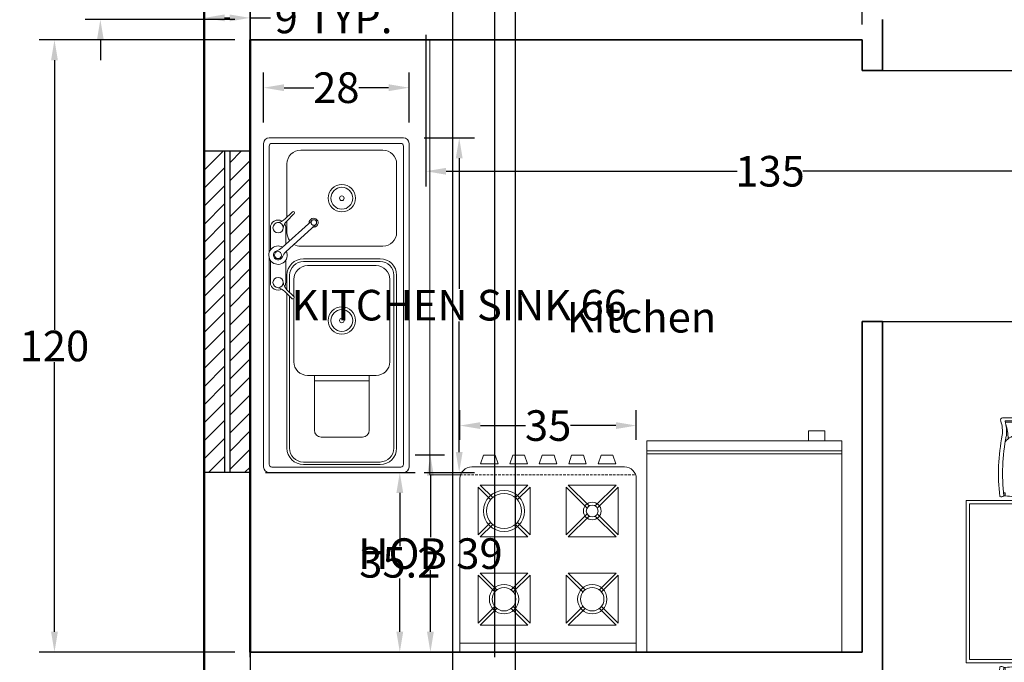
# Model space of a CAD drawing. Units: inches. Extents: x -1285 to -837, y -84 to 552.
# Tile 2 of 10: x -1282 to -1089, y 38 to 164. Entities that reach past the tile are written whole.
import ezdxf

# ---------------------------------------------------------------- set-up
doc = ezdxf.new("R2010")
doc.units = ezdxf.units.IN
doc.header["$MEASUREMENT"] = 0
doc.linetypes.add('DASHED', pattern=[0.75, 0.5, -0.25])
for name, color, linetype, lineweight in [('A-ANNO-DIMS', 2, 'Continuous', 18), ('A-AREA-IDEN', 7, 'Continuous', 25), ('A-FURN-CSWK', 9, 'Continuous', 18), ('A-FURN-CSWK-HIDN', 9, 'DASHED', 13), ('A-GLAZ-PATT', 191, 'Continuous', 13), ('Dining Table', 52, 'Continuous', 18), ('Gas Stove', 31, 'Continuous', 18), ('Inner Wall', 202, 'Continuous', 35), ('Outer Wall', 12, 'Continuous', 50), ('Refrigerator', 8, 'Continuous', 18), ('Sink', 33, 'Continuous', 18), ('Windows', 191, 'Continuous', 25)]:
    doc.layers.add(name, color=color, linetype=linetype, lineweight=lineweight)
doc.styles.get("Standard").update_dxf_attribs({"font": 'arial.ttf'})
doc.dimstyles.get("Standard").update_dxf_attribs({"dimtxt": 6, "dimasz": 4, "dimexe": 3, "dimexo": 3, "dimgap": 0.09, "dimtad": 0, "dimtih": 1, "dimtoh": 1, "dimdec": 1, "dimzin": 0, "dimdsep": 46, "dimlunit": 3, "dimtxsty": 'Standard', "dimcen": 0.09, "dimadec": 0, "dimazin": 0, "dimtfac": 1, "dimtdec": 1, "dimtofl": 0, "dimtmove": 0, "dimatfit": 3, "dimfxl": 1, "dimtolj": 1, "dimtzin": 0, "dimarcsym": 0})

# ---------------------------------------------------------------- blocks, each defined once
blk = doc.blocks.new('Gas Stove')
at = {"color": 0}
for p, q in [((1658.63, 622.25), (1657.94, 620.18)), ((1658.63, 622.25), (1661.39, 622.25)), ((1661.39, 622.25), (1662.08, 620.18)), ((1665.52, 622.25), (1664.83, 620.18)), ((1665.52, 622.25), (1668.27, 622.25)), ((1668.27, 622.25), (1668.96, 620.18)), ((1672.4, 622.25), (1671.72, 620.18)), ((1672.4, 622.25), (1675.16, 622.25)), ((1675.16, 622.25), (1675.85, 620.18)), ((1679.29, 622.25), (1678.6, 620.18)), ((1679.29, 622.25), (1682.04, 622.25)), ((1682.04, 622.25), (1682.73, 620.18)), ((1686.18, 622.25), (1685.49, 620.18)), ((1686.18, 622.25), (1688.93, 622.25)), ((1688.93, 622.25), (1689.62, 620.18)), ((1655.88, 619.49), (1691.68, 619.49)), ((1657.94, 620.18), (1662.08, 620.18)), ((1664.83, 620.18), (1668.96, 620.18)), ((1671.72, 620.18), (1675.85, 620.18)), ((1678.6, 620.18), (1682.73, 620.18)), ((1685.49, 620.18), (1689.62, 620.18)), ((1653.12, 576.11), (1653.12, 616.74)), ((1694.44, 616.74), (1694.44, 576.11)), ((1657.37, 603.57), (1657.37, 614.76)), ((1660.3, 611.83), (1657.37, 614.76)), ((1657.85, 615.25), (1669.05, 615.25)), ((1660.79, 612.32), (1657.85, 615.25)), ((1666.12, 612.32), (1669.05, 615.25)), ((1666.61, 611.83), (1669.54, 614.76)), ((1669.54, 614.76), (1669.54, 603.57)), ((1678.02, 603.57), (1678.02, 614.76)), ((1678.02, 614.76), (1682.92, 609.86)), ((1678.51, 615.25), (1689.71, 615.25)), ((1678.51, 615.25), (1683.41, 610.35)), ((1684.81, 610.35), (1689.71, 615.25)), ((1685.3, 609.86), (1690.2, 614.76)), ((1690.2, 614.76), (1690.2, 603.57)), ((1678.02, 603.57), (1682.92, 608.47)), ((1678.51, 603.08), (1683.41, 607.98)), ((1684.81, 607.98), (1689.71, 603.08)), ((1685.3, 608.47), (1690.2, 603.57)), ((1657.37, 603.57), (1660.3, 606.5)), ((1657.85, 603.08), (1660.79, 606.01)), ((1669.05, 603.08), (1666.12, 606.01)), ((1669.54, 603.57), (1666.61, 606.5)), ((1669.05, 603.08), (1657.85, 603.08)), ((1689.71, 603.08), (1678.51, 603.08)), ((1657.37, 582.91), (1657.37, 594.11)), ((1661.28, 590.2), (1657.37, 594.11)), ((1657.85, 594.59), (1669.05, 594.59)), ((1661.76, 590.68), (1657.85, 594.59)), ((1669.05, 594.59), (1665.14, 590.68)), ((1669.54, 594.11), (1665.63, 590.2)), ((1669.54, 594.11), (1669.54, 582.91)), ((1678.02, 582.91), (1678.02, 594.11)), ((1678.02, 594.11), (1681.93, 590.2)), ((1678.51, 594.59), (1689.71, 594.59)), ((1678.51, 594.59), (1682.42, 590.68)), ((1689.71, 594.59), (1685.8, 590.68)), ((1690.2, 594.11), (1686.29, 590.2)), ((1690.2, 594.11), (1690.2, 582.91)), ((1661.28, 586.82), (1657.37, 582.91)), ((1661.76, 586.33), (1657.85, 582.42)), ((1669.05, 582.42), (1665.14, 586.33)), ((1669.54, 582.91), (1665.63, 586.82)), ((1681.93, 586.82), (1678.02, 582.91)), ((1682.42, 586.33), (1678.51, 582.42)), ((1685.8, 586.33), (1689.71, 582.42)), ((1686.29, 586.82), (1690.2, 582.91)), ((1669.05, 582.42), (1657.85, 582.42)), ((1689.71, 582.42), (1678.51, 582.42)), ((1694.44, 578.18), (1653.12, 578.18)), ((1694.44, 576.11), (1653.12, 576.11))]:
    blk.add_line(p, q, dxfattribs=at)
for centre, radius in [((1663.45, 609.16), 4.82), ((1663.45, 609.16), 4.13), ((1684.11, 609.16), 2.07), ((1684.11, 609.16), 1.38), ((1663.45, 588.51), 3.44), ((1663.45, 588.51), 2.75), ((1684.11, 588.51), 3.44), ((1684.11, 588.51), 2.75)]:
    blk.add_circle(centre, radius, dxfattribs=at)
for centre, start, end in [((1655.88, 616.74), 90, 180), ((1691.68, 616.74), 0, 90)]:
    blk.add_arc(centre, 2.75, start, end, dxfattribs=at)
blk = doc.blocks.new('Kitchen Sink')
at = {"color": 0}
for p, q in [((789.24, 1687.8), (613.32, 1687.8)), ((610.34, 1684.82), (610.34, 1611.77)), ((613.32, 1683.33), (613.32, 1613.26)), ((727.2, 1684.82), (614.81, 1684.82)), ((725.7, 1684.14), (713.58, 1684.14)), ((787.75, 1684.82), (729.77, 1684.82)), ((743.4, 1684.14), (731.28, 1684.14)), ((789.24, 1613.26), (789.24, 1683.33)), ((792.22, 1684.82), (792.22, 1611.77)), ((708.68, 1676.2), (705.1, 1672.69)), ((725.7, 1675.81), (713.58, 1675.81)), ((730.36, 1675.71), (745.02, 1659.62)), ((732.56, 1677.72), (747.22, 1661.63)), ((743.4, 1675.81), (734.3, 1675.81)), ((748.23, 1676.11), (751.75, 1672.54)), ((707.58, 1675.13), (623.63, 1675.13)), ((706.19, 1673.76), (623.63, 1673.76)), ((670.59, 1671.4), (704.9, 1671.4)), ((705.98, 1671.4), (715.32, 1671.4)), ((709.72, 1675.14), (706.14, 1671.62)), ((717.55, 1673.76), (708.32, 1673.76)), ((717.55, 1675.13), (709.71, 1675.13)), ((740.79, 1675.13), (747.11, 1675.13)), ((747.17, 1675.07), (750.68, 1671.49)), ((749.2, 1675.13), (778.06, 1675.13)), ((614.69, 1666.18), (614.69, 1624.44)), ((616.05, 1666.18), (616.05, 1624.44)), ((725.01, 1624.44), (725.01, 1666.18)), ((726.5, 1624.44), (726.5, 1666.18)), ((733.33, 1622.95), (733.33, 1667.67)), ((785.51, 1622.95), (785.51, 1667.67)), ((663.14, 1660.22), (633.32, 1660.22)), ((660.16, 1630.4), (660.16, 1660.22)), ((663.14, 1626.68), (663.14, 1663.95)), ((722.77, 1626.68), (722.77, 1663.95)), ((629.6, 1656.49), (629.6, 1634.13)), ((663.14, 1630.4), (633.32, 1630.4)), ((623.63, 1616.99), (717.55, 1616.99)), ((670.59, 1619.22), (715.32, 1619.22)), ((614.81, 1611.77), (787.75, 1611.77)), ((623.63, 1615.5), (717.55, 1615.5)), ((740.79, 1615.5), (778.06, 1615.5)), ((613.32, 1608.79), (789.24, 1608.79))]:
    blk.add_line(p, q, dxfattribs=at)
for centre, radius in [((713.58, 1679.97), 2.79), ((728.49, 1679.97), 1.91), ((743.4, 1679.97), 2.79), ((746.22, 1660.52), 1.5), ((692.96, 1645.31), 7.45), ((692.96, 1645.31), 5.96), ((759.42, 1645.31), 7.45), ((759.42, 1645.31), 5.96), ((692.96, 1645.31), 1.27), ((759.42, 1645.31), 1.27)]:
    blk.add_circle(centre, radius, dxfattribs=at)
for centre, radius, start, end in [((613.32, 1684.82), 2.98, 90, 180), ((789.24, 1684.82), 2.98, 0, 90), ((614.81, 1683.33), 1.49, 90, 180), ((713.58, 1679.97), 4.17, 90, 209.8816), ((728.49, 1679.97), 5.01, 329.6444, 295.0423), ((728.49, 1679.97), 2.52, 16.0755, 248.6112), ((738.07, 1682.74), 7.45, 196.0755, 222.3434), ((743.4, 1679.97), 4.17, 329.1097, 90), ((787.75, 1683.33), 1.49, 0, 90), ((703.45, 1681.52), 7.45, 314.4956, 351.339), ((714.94, 1669.82), 7.45, 97.6523, 134.4956), ((713.58, 1679.97), 4.17, 239.1097, 270), ((724.85, 1670.69), 7.45, 42.3434, 68.6112), ((741.85, 1669.84), 7.45, 44.4956, 81.339), ((743.4, 1679.97), 4.17, 270, 299.8816), ((753.55, 1681.34), 7.45, 187.6523, 224.4956), ((623.63, 1666.18), 8.94, 90, 180), ((623.63, 1666.18), 7.58, 90, 180), ((670.59, 1663.95), 7.45, 90, 180), ((670.59, 1663.95), 7.45, 90, 91.1456), ((705.44, 1671.98), 0.787, 115.7239, 333.2674), ((715.32, 1663.95), 7.45, 0, 90), ((717.55, 1666.18), 8.94, 0, 90), ((717.34, 1666.09), 7.67, 0.6729, 88.3753), ((740.79, 1667.67), 7.45, 150.2915, 180), ((740.79, 1667.67), 7.45, 90, 127.0737), ((751.39, 1671.84), 0.787, 205.7239, 63.2674), ((778.06, 1667.67), 7.45, 0, 90), ((633.32, 1656.49), 3.73, 90, 180), ((746.12, 1660.63), 2.42, 170.3658, 94.3209), ((633.32, 1634.13), 3.73, 180, 270), ((623.63, 1624.44), 8.94, 180, 270), ((623.72, 1624.66), 7.67, 181.6247, 269.3271), ((670.59, 1626.68), 7.45, 180, 270), ((715.32, 1626.68), 7.45, 270, 0), ((717.55, 1624.44), 8.94, 270, 0), ((717.55, 1624.44), 7.45, 270, 0), ((740.79, 1622.95), 7.45, 180, 270), ((778.06, 1622.95), 7.45, 270, 0), ((613.32, 1611.77), 2.98, 180, 270), ((614.81, 1613.26), 1.49, 180, 270), ((787.75, 1613.26), 1.49, 270, 0), ((789.24, 1611.77), 2.98, 270, 0)]:
    blk.add_arc(centre, radius, start, end, dxfattribs=at)
blk = doc.blocks.new('A$C51F1')
at = {"color": 0}
for p, q in [((0.2273, 0.4758), (0.0436, 0.4758)), ((0.2273, 0.4676), (0.0439, 0.4676)), ((0.2273, 0.4668), (0.0439, 0.4668)), ((0.2273, 0.4758), (0.4111, 0.4758)), ((0.2273, 0.4676), (0.4107, 0.4676)), ((0.2273, 0.4668), (0.4107, 0.4668)), ((0.2273, 0.3858), (0.1205, 0.3858)), ((0.2273, 0.3858), (0.3341, 0.3858)), ((0.0417, 0.0321), (0.0321, 0.0321)), ((0.0417, 0.0321), (0.0326, 0.0278)), ((0.0435, 0.0127), (0.0417, 0.0321)), ((0.4112, 0.0127), (0.4129, 0.0321)), ((0.4129, 0.0321), (0.4225, 0.0321)), ((0.4129, 0.0321), (0.4221, 0.0278))]:
    blk.add_line(p, q, dxfattribs=at)
blk.add_lwpolyline([(0.4387, 0.4737, 0.102523), (0.4291, 0.3863, -0.080461), (0.4447, 0.0091, -0.3023), (0.4203, 0.012, 0.197932), (0.4111, 0.0127, -0.028193), (0.3571, 0.0091), (0.227, 0.0091), (0.097, 0.0091, -0.028193), (0.0429, 0.0127, 0.197932), (0.0338, 0.012, -0.3023), (0.0093, 0.0091, -0.080461), (0.0249, 0.3863, 0.102523), (0.0153, 0.4737, -0.587111), (0.0261, 0.4929), (0.4279, 0.4929, -0.587111)], format="xyb", close=True, dxfattribs=at)
for centre, radius, start, end in [((0.044, 0.4735), 0.00242, 100.34496, 201.37417), ((-0.1898, 0.4063), 0.2409, 354.55133, 15.96258), ((0.0439, 0.4669), 0.000725, 87.37617, 197.52085), ((0.0438, 0.4664), 0.000433, 71.7715, 189.22024), ((-0.2563, 0.3584), 0.3173, 1.15909, 17.56409), ((0.7109, 0.3584), 0.3173, 162.43591, 178.84091), ((0.6445, 0.4063), 0.2409, 164.03742, 185.44867), ((0.4107, 0.4669), 0.000725, 342.47915, 92.62383), ((0.4109, 0.4664), 0.000433, 350.77976, 108.2285), ((0.4106, 0.4735), 0.00242, 338.62583, 79.65504), ((1.1806, 0.1494), 1.1544, 168.43567, 186.83625), ((0.1214, 0.2879), 0.0978, 90.51639, 143.19267), ((0.3332, 0.2879), 0.0978, 36.80733, 89.48361), ((-0.7259, 0.1494), 1.1544, 353.16375, 11.56433), ((0.0397, 0.0013), 0.012, 71.75361, 116.5375), ((0.4149, 0.0013), 0.012, 63.4625, 108.24639)]:
    blk.add_arc(centre, radius, start, end, dxfattribs=at)
blk = doc.blocks.new('Dining Table')
at = {"color": 0, "ltscale": 0.5}
for points in [[(5887.4, 1648.9), (7887.4, 1648.9), (7887.4, 2648.9), (5887.4, 2648.9)], [(5907.4, 1668.9), (7867.4, 1668.9), (7867.4, 2628.9), (5907.4, 2628.9)]]:
    blk.add_lwpolyline(points, close=True, dxfattribs=at)
at = {"color": 0, "ltscale": 0.5, "yscale": 1000, "zscale": 1000}
for p, xscale in [((6085.4, 2664.8), 1000), ((6685.4, 2664.8), 1000), ((7739.4, 2664.8), -1000)]:
    blk.add_blockref('A$C51F1', p, dxfattribs=dict(at, xscale=xscale))
at = {"color": 0, "ltscale": 0.5, "yscale": 1000, "zscale": 1000, "rotation": 180}
for p, xscale in [((6085.4, 1633), -1000), ((6685.4, 1633), -1000), ((7739.4, 1633), 1000)]:
    blk.add_blockref('A$C51F1', p, dxfattribs=dict(at, xscale=xscale))
blk = doc.blocks.new('WIN-63x9')
for p, q in [((4, 63.04), (4, 0)), ((5, 63.04), (5, 0))]:
    blk.add_line(p, q)
blk.add_lwpolyline([(0, 0), (0, 63.04), (9, 63.04), (9, 0)], close=True)
blk = doc.blocks.new('*D34')
at = {"layer": 'A-ANNO-DIMS', "color": 0, "lineweight": -2, "transparency": 16777216}
for p, q in [((-1245.53, 166.4), (-1245.53, 161.25)), ((-1236.53, 166.4), (-1236.53, 161.25)), ((-1241.53, 164.25), (-1240.53, 164.25)), ((-1236.53, 164.25), (-1232.53, 164.25))]:
    blk.add_line(p, q, dxfattribs=at)
at = {"layer": 'A-ANNO-DIMS', "color": 0, "transparency": 16777216}
for points in [[(-1241.53, 164.92), (-1241.53, 163.58), (-1245.53, 164.25)], [(-1240.53, 164.92), (-1240.53, 163.58), (-1236.53, 164.25)]]:
    blk.add_solid(points, dxfattribs=at)
at = {"layer": 'Defpoints', "color": 0, "transparency": 16777216}
for p in [(-1245.53, 169.4), (-1236.53, 169.4), (-1236.53, 164.25)]:
    blk.add_point(p, dxfattribs=at)
at = {"layer": 'A-ANNO-DIMS', "color": 0, "transparency": 16777216, "insert": (-1220.17, 164.25), "char_height": 6, "attachment_point": 5}
blk.add_mtext('\\A1;9 TYP.', dxfattribs=at)
blk = doc.blocks.new('*D49')
at = {"layer": 'A-ANNO-DIMS', "color": 0, "lineweight": -2, "transparency": 16777216}
for p, q in [((-1198.39, 78.55), (-1204.18, 78.55)), ((-1201.18, 74.55), (-1201.18, 62.44)), ((-1201.18, 43.94), (-1201.18, 56.05)), ((-1198.39, 39.94), (-1204.18, 39.94))]:
    blk.add_line(p, q, dxfattribs=at)
at = {"layer": 'A-ANNO-DIMS', "color": 0, "transparency": 16777216}
for points in [[(-1201.85, 74.55), (-1200.51, 74.55), (-1201.18, 78.55)], [(-1201.85, 43.94), (-1200.51, 43.94), (-1201.18, 39.94)]]:
    blk.add_solid(points, dxfattribs=at)
at = {"layer": 'Defpoints', "color": 0, "transparency": 16777216}
for p in [(-1201.18, 78.55), (-1195.39, 78.55), (-1195.39, 39.94)]:
    blk.add_point(p, dxfattribs=at)
at = {"layer": 'A-ANNO-DIMS', "color": 0, "transparency": 16777216, "insert": (-1201.18, 59.24), "char_height": 6, "attachment_point": 5}
blk.add_mtext('\\A1;HOB 39', dxfattribs=at)
blk = doc.blocks.new('*D50')
at = {"layer": 'A-ANNO-DIMS', "color": 0, "lineweight": -2, "transparency": 16777216}
for p, q in [((-1195.39, 81.55), (-1195.39, 87.34)), ((-1160.81, 81.55), (-1160.81, 87.34)), ((-1191.39, 84.34), (-1182.51, 84.34)), ((-1164.81, 84.34), (-1173.69, 84.34))]:
    blk.add_line(p, q, dxfattribs=at)
at = {"layer": 'A-ANNO-DIMS', "color": 0, "transparency": 16777216}
for points in [[(-1191.39, 85.01), (-1191.39, 83.67), (-1195.39, 84.34)], [(-1164.81, 85.01), (-1164.81, 83.67), (-1160.81, 84.34)]]:
    blk.add_solid(points, dxfattribs=at)
at = {"layer": 'Defpoints', "color": 0, "transparency": 16777216}
for p in [(-1160.81, 84.34), (-1195.39, 78.55), (-1160.81, 78.55)]:
    blk.add_point(p, dxfattribs=at)
at = {"layer": 'A-ANNO-DIMS', "color": 0, "transparency": 16777216, "insert": (-1178.1, 84.34), "char_height": 6, "attachment_point": 5}
blk.add_mtext('\\A1;35', dxfattribs=at)
blk = doc.blocks.new('*D51')
at = {"layer": 'A-ANNO-DIMS', "color": 0, "lineweight": -2, "transparency": 16777216}
for p, q in [((-1202.37, 140.73), (-1192.53, 140.73)), ((-1195.53, 136.73), (-1195.53, 111.13)), ((-1195.53, 79.14), (-1195.53, 104.74)), ((-1202.37, 75.14), (-1192.53, 75.14))]:
    blk.add_line(p, q, dxfattribs=at)
at = {"layer": 'A-ANNO-DIMS', "color": 0, "transparency": 16777216}
for points in [[(-1196.2, 136.73), (-1194.87, 136.73), (-1195.53, 140.73)], [(-1196.2, 79.14), (-1194.87, 79.14), (-1195.53, 75.14)]]:
    blk.add_solid(points, dxfattribs=at)
at = {"layer": 'Defpoints', "color": 0, "transparency": 16777216}
for p in [(-1205.37, 140.73), (-1195.53, 140.73), (-1205.37, 75.14)]:
    blk.add_point(p, dxfattribs=at)
at = {"layer": 'A-ANNO-DIMS', "color": 0, "transparency": 16777216, "insert": (-1195.53, 107.94), "char_height": 6, "attachment_point": 5}
blk.add_mtext('\\A1;KITCHEN SINK 66', dxfattribs=at)
blk = doc.blocks.new('*D52')
at = {"layer": 'A-ANNO-DIMS', "color": 0, "lineweight": -2, "transparency": 16777216}
for p, q in [((-1233.87, 143.73), (-1233.87, 153.57)), ((-1205.37, 143.73), (-1205.37, 153.57)), ((-1229.87, 150.57), (-1224.06, 150.57)), ((-1209.37, 150.57), (-1215.18, 150.57))]:
    blk.add_line(p, q, dxfattribs=at)
at = {"layer": 'A-ANNO-DIMS', "color": 0, "transparency": 16777216}
for points in [[(-1229.87, 151.24), (-1229.87, 149.9), (-1233.87, 150.57)], [(-1209.37, 151.24), (-1209.37, 149.9), (-1205.37, 150.57)]]:
    blk.add_solid(points, dxfattribs=at)
at = {"layer": 'Defpoints', "color": 0, "transparency": 16777216}
for p in [(-1233.87, 150.57), (-1233.87, 140.73), (-1205.37, 140.73)]:
    blk.add_point(p, dxfattribs=at)
at = {"layer": 'A-ANNO-DIMS', "color": 0, "transparency": 16777216, "insert": (-1219.62, 150.57), "char_height": 6, "attachment_point": 5}
blk.add_mtext('\\A1;28', dxfattribs=at)
blk = doc.blocks.new('*D66')
at = {"layer": 'A-ANNO-DIMS', "color": 0, "lineweight": -2, "transparency": 16777216}
for p, q in [((-1202.09, 160.9), (-1202.09, 131.19)), ((-1067.13, 160.9), (-1067.13, 131.19)), ((-1198.09, 134.19), (-1141.07, 134.19)), ((-1071.13, 134.19), (-1128.15, 134.19))]:
    blk.add_line(p, q, dxfattribs=at)
at = {"layer": 'A-ANNO-DIMS', "color": 0, "transparency": 16777216}
for points in [[(-1198.09, 134.86), (-1198.09, 133.52), (-1202.09, 134.19)], [(-1071.13, 134.86), (-1071.13, 133.52), (-1067.13, 134.19)]]:
    blk.add_solid(points, dxfattribs=at)
at = {"layer": 'Defpoints', "color": 0, "transparency": 16777216}
for p in [(-1202.09, 163.9), (-1067.13, 163.9), (-1067.13, 134.19)]:
    blk.add_point(p, dxfattribs=at)
at = {"layer": 'A-ANNO-DIMS', "color": 0, "transparency": 16777216, "insert": (-1134.61, 134.19), "char_height": 6, "attachment_point": 5}
blk.add_mtext('\\A1;135', dxfattribs=at)
blk = doc.blocks.new('*D76')
at = {"layer": 'A-ANNO-DIMS', "color": 0, "lineweight": -2, "transparency": 16777216}
for p, q in [((-1239.53, 159.94), (-1277.88, 159.94)), ((-1274.88, 155.94), (-1274.88, 103.09)), ((-1274.88, 43.94), (-1274.88, 96.79)), ((-1239.53, 39.94), (-1277.88, 39.94))]:
    blk.add_line(p, q, dxfattribs=at)
at = {"layer": 'A-ANNO-DIMS', "color": 0, "transparency": 16777216}
for points in [[(-1275.55, 155.94), (-1274.21, 155.94), (-1274.88, 159.94)], [(-1275.55, 43.94), (-1274.21, 43.94), (-1274.88, 39.94)]]:
    blk.add_solid(points, dxfattribs=at)
at = {"layer": 'Defpoints', "color": 0, "transparency": 16777216}
for p in [(-1274.88, 159.94), (-1236.53, 159.94), (-1236.53, 39.94)]:
    blk.add_point(p, dxfattribs=at)
at = {"layer": 'A-ANNO-DIMS', "color": 0, "transparency": 16777216, "insert": (-1274.88, 99.94), "char_height": 6, "attachment_point": 5}
blk.add_mtext('\\A1;120', dxfattribs=at)
blk = doc.blocks.new('*D78')
at = {"layer": 'A-ANNO-DIMS', "color": 0, "lineweight": -2, "transparency": 16777216}
for p, q in [((-1236.53, 162.94), (-1236.53, 551.29)), ((-1116.53, 162.94), (-1116.53, 551.29)), ((-1232.53, 548.29), (-1182.96, 548.29)), ((-1120.53, 548.29), (-1170.1, 548.29))]:
    blk.add_line(p, q, dxfattribs=at)
at = {"layer": 'A-ANNO-DIMS', "color": 0, "transparency": 16777216}
for points in [[(-1232.53, 548.96), (-1232.53, 547.62), (-1236.53, 548.29)], [(-1120.53, 548.96), (-1120.53, 547.62), (-1116.53, 548.29)]]:
    blk.add_solid(points, dxfattribs=at)
at = {"layer": 'Defpoints', "color": 0, "transparency": 16777216}
for p in [(-1116.53, 548.29), (-1236.53, 159.94), (-1116.53, 159.94)]:
    blk.add_point(p, dxfattribs=at)
at = {"layer": 'A-ANNO-DIMS', "color": 0, "transparency": 16777216, "insert": (-1176.53, 548.29), "char_height": 6, "attachment_point": 5}
blk.add_mtext('\\A1;120', dxfattribs=at)
blk = doc.blocks.new('*D79')
at = {"layer": 'A-ANNO-DIMS', "color": 0, "lineweight": -2, "transparency": 16777216}
for p, q in [((-1236.53, 38.94), (-1236.53, 551.29)), ((-1188.53, 38.94), (-1188.53, 551.29)), ((-1232.53, 548.29), (-1217.04, 548.29)), ((-1192.53, 548.29), (-1208.02, 548.29))]:
    blk.add_line(p, q, dxfattribs=at)
at = {"layer": 'A-ANNO-DIMS', "color": 0, "transparency": 16777216}
for points in [[(-1232.53, 548.96), (-1232.53, 547.62), (-1236.53, 548.29)], [(-1192.53, 548.96), (-1192.53, 547.62), (-1188.53, 548.29)]]:
    blk.add_solid(points, dxfattribs=at)
at = {"layer": 'Defpoints', "color": 0, "transparency": 16777216}
for p in [(-1188.53, 548.29), (-1236.53, 35.94), (-1188.53, 35.94)]:
    blk.add_point(p, dxfattribs=at)
at = {"layer": 'A-ANNO-DIMS', "color": 0, "transparency": 16777216, "insert": (-1212.53, 548.29), "char_height": 6, "attachment_point": 5}
blk.add_mtext('\\A1;48', dxfattribs=at)
blk = doc.blocks.new('*D80')
at = {"layer": 'A-ANNO-DIMS', "color": 0, "lineweight": -2, "transparency": 16777216}
for p, q in [((-1184.53, -13.66), (-1184.53, 551.29)), ((-1032.53, -13.66), (-1032.53, 551.29)), ((-1180.53, 548.29), (-1114.94, 548.29)), ((-1036.53, 548.29), (-1102.12, 548.29))]:
    blk.add_line(p, q, dxfattribs=at)
at = {"layer": 'A-ANNO-DIMS', "color": 0, "transparency": 16777216}
for points in [[(-1180.53, 548.96), (-1180.53, 547.62), (-1184.53, 548.29)], [(-1036.53, 548.96), (-1036.53, 547.62), (-1032.53, 548.29)]]:
    blk.add_solid(points, dxfattribs=at)
at = {"layer": 'Defpoints', "color": 0, "transparency": 16777216}
for p in [(-1032.53, 548.29), (-1184.53, -16.66), (-1032.53, -16.66)]:
    blk.add_point(p, dxfattribs=at)
at = {"layer": 'A-ANNO-DIMS', "color": 0, "transparency": 16777216, "insert": (-1108.53, 548.29), "char_height": 6, "attachment_point": 5}
blk.add_mtext('\\A1;152', dxfattribs=at)
blk = doc.blocks.new('*D92')
at = {"layer": 'A-ANNO-DIMS', "color": 0, "lineweight": -2, "transparency": 16777216}
for p, q in [((-1113.53, 153.94), (-845.18, 153.94)), ((-848.18, 149.94), (-848.18, 132.48)), ((-848.18, 108.72), (-848.18, 126.18)), ((-1113.53, 104.72), (-845.18, 104.72))]:
    blk.add_line(p, q, dxfattribs=at)
at = {"layer": 'A-ANNO-DIMS', "color": 0, "transparency": 16777216}
for points in [[(-848.85, 149.94), (-847.51, 149.94), (-848.18, 153.94)], [(-848.85, 108.72), (-847.51, 108.72), (-848.18, 104.72)]]:
    blk.add_solid(points, dxfattribs=at)
at = {"layer": 'Defpoints', "color": 0, "transparency": 16777216}
for p in [(-1116.53, 153.94), (-848.18, 153.94), (-1116.53, 104.72)]:
    blk.add_point(p, dxfattribs=at)
at = {"layer": 'A-ANNO-DIMS', "color": 0, "transparency": 16777216, "insert": (-848.18, 129.33), "char_height": 6, "attachment_point": 5}
blk.add_mtext('\\A1;49.22', dxfattribs=at)
blk = doc.blocks.new('*D96')
at = {"layer": 'A-ANNO-DIMS', "color": 0, "lineweight": -2, "transparency": 16777216}
for p, q in [((-1236.53, 506.94), (-1236.53, -83.53)), ((-1196.84, 506.94), (-1196.84, -83.53)), ((-1232.53, -80.53), (-1226.9, -80.53)), ((-1200.84, -80.53), (-1206.47, -80.53))]:
    blk.add_line(p, q, dxfattribs=at)
at = {"layer": 'A-ANNO-DIMS', "color": 0, "transparency": 16777216}
for points in [[(-1232.53, -79.86), (-1232.53, -81.2), (-1236.53, -80.53)], [(-1200.84, -79.86), (-1200.84, -81.2), (-1196.84, -80.53)]]:
    blk.add_solid(points, dxfattribs=at)
at = {"layer": 'Defpoints', "color": 0, "transparency": 16777216}
for p in [(-1236.53, 509.94), (-1196.84, 509.94), (-1196.84, -80.53)]:
    blk.add_point(p, dxfattribs=at)
at = {"layer": 'A-ANNO-DIMS', "color": 0, "transparency": 16777216, "insert": (-1216.68, -80.53), "char_height": 6, "attachment_point": 5}
blk.add_mtext('\\A1;39.69', dxfattribs=at)
blk = doc.blocks.new('*D99')
at = {"layer": 'A-ANNO-DIMS', "color": 0, "lineweight": -2, "transparency": 16777216}
for p, q in [((-1233.53, 75.14), (-1204.18, 75.14)), ((-1207.18, 71.14), (-1207.18, 60.69)), ((-1207.18, 43.94), (-1207.18, 54.38)), ((-1233.53, 39.94), (-1204.18, 39.94))]:
    blk.add_line(p, q, dxfattribs=at)
at = {"layer": 'A-ANNO-DIMS', "color": 0, "transparency": 16777216}
for points in [[(-1207.85, 71.14), (-1206.51, 71.14), (-1207.18, 75.14)], [(-1207.85, 43.94), (-1206.51, 43.94), (-1207.18, 39.94)]]:
    blk.add_solid(points, dxfattribs=at)
at = {"layer": 'Defpoints', "color": 0, "transparency": 16777216}
for p in [(-1236.53, 75.14), (-1236.53, 39.94), (-1207.18, 39.94)]:
    blk.add_point(p, dxfattribs=at)
at = {"layer": 'A-ANNO-DIMS', "color": 0, "transparency": 16777216, "insert": (-1207.18, 57.54), "char_height": 6, "attachment_point": 5}
blk.add_mtext('\\A1;35.2', dxfattribs=at)
blk = doc.blocks.new('*D113')
at = {"layer": 'A-ANNO-DIMS', "color": 0, "lineweight": -2, "transparency": 16777216}
for p, q in [((-1265.88, 173.4), (-1265.88, 177.4)), ((-1265.88, 177.4), (-1261.88, 177.4)), ((-1239.53, 169.4), (-1268.88, 169.4)), ((-1239.53, 163.94), (-1268.88, 163.94)), ((-1265.88, 159.94), (-1265.88, 155.94))]:
    blk.add_line(p, q, dxfattribs=at)
at = {"layer": 'A-ANNO-DIMS', "color": 0, "transparency": 16777216}
for points in [[(-1266.55, 173.4), (-1265.21, 173.4), (-1265.88, 169.4)], [(-1266.55, 159.94), (-1265.21, 159.94), (-1265.88, 163.94)]]:
    blk.add_solid(points, dxfattribs=at)
at = {"layer": 'Defpoints', "color": 0, "transparency": 16777216}
for p in [(-1265.88, 169.4), (-1236.53, 169.4), (-1236.53, 163.94)]:
    blk.add_point(p, dxfattribs=at)
at = {"layer": 'A-ANNO-DIMS', "color": 0, "transparency": 16777216, "insert": (-1251.68, 177.4), "char_height": 6, "attachment_point": 5}
blk.add_mtext('\\A1;5.464', dxfattribs=at)

msp = doc.modelspace()

# ---------------------------------------------------------------- hatches: boundary and pattern name
at = {"layer": 'A-GLAZ-PATT'}
h = msp.add_hatch(dxfattribs=at)
h.set_pattern_fill('ANSI31', color=256, scale=20)
h.set_pattern_definition([(45, (-2191.666, -702.1458), (-1.767767, 1.767767), [])])
h.paths.add_polyline_path([(-921.1945, 518.9392), (-984.2307, 518.9392), (-984.2307, 514.9392), (-921.1945, 514.9392)])
h.paths.add_polyline_path([(-921.1945, 513.9392), (-984.2307, 513.9392), (-984.2307, 509.9392), (-921.1945, 509.9392)])
h.paths.add_polyline_path([(-877.5299, 480.0491), (-881.5299, 480.0491), (-881.5299, 417.0129), (-877.5299, 417.0129)])
h.paths.add_polyline_path([(-882.5299, 480.0491), (-886.5299, 480.0491), (-886.5299, 417.0129), (-882.5299, 417.0129)])
h.paths.add_polyline_path([(-877.5299, 356.1195), (-881.5299, 356.1195), (-881.5299, 321.7709), (-877.5299, 321.7709)])
h.paths.add_polyline_path([(-882.5299, 356.1195), (-886.5299, 356.1195), (-886.5299, 321.7709), (-882.5299, 321.7709)])
h.paths.add_polyline_path([(-1133.8033, 518.9392), (-1196.8396, 518.9392), (-1196.8396, 514.9392), (-1133.8033, 514.9392)])
h.paths.add_polyline_path([(-1133.8033, 513.9392), (-1196.8396, 513.9392), (-1196.8396, 509.9392), (-1133.8033, 509.9392)])
h.paths.add_polyline_path([(-1236.5299, 138.1751), (-1240.5299, 138.1751), (-1240.5299, 75.1388), (-1236.5299, 75.1388)])
h.paths.add_polyline_path([(-1241.5299, 138.1751), (-1245.5299, 138.1751), (-1245.5299, 75.1388), (-1241.5299, 75.1388)])
h.paths.add_polyline_path([(-1236.5299, 35.9392), (-1240.5299, 35.9392), (-1240.5299, 1.5906), (-1236.5299, 1.5906)])
h.paths.add_polyline_path([(-1241.5299, 35.9392), (-1245.5299, 35.9392), (-1245.5299, 1.5906), (-1241.5299, 1.5906)])
h.paths.add_polyline_path([(-1088.8155, -16.6608), (-1136.8155, -16.6608), (-1136.8155, -20.6608), (-1088.8155, -20.6608)])
h.paths.add_polyline_path([(-1088.8155, -21.6608), (-1136.8155, -21.6608), (-1136.8155, -25.6608), (-1088.8155, -25.6608)])

# ---------------------------------------------------------------- linework, layer by layer
at = {"layer": 'A-FURN-CSWK'}
for p, q in [((-1201.306, 159.9392), (-1201.306, 74.703)), ((-1201.306, 74.703), (-1195.3885, 74.703))]:
    msp.add_line(p, q, dxfattribs=at)
at = {"layer": 'A-FURN-CSWK-HIDN'}
msp.add_line((-1195.3885, 74.703), (-1160.9424, 74.703), dxfattribs=at)
at = {"layer": 'Inner Wall'}
for p, q in [((-1112.5299, 163.9392), (-1112.5299, 153.9392)), ((-1236.5299, 159.9392), (-1116.5299, 159.9392)), ((-1116.5299, 159.9392), (-1116.5299, 153.9392)), ((-1116.5299, 153.9392), (-1112.5299, 153.9392)), ((-1116.5299, 104.7212), (-1116.5299, 39.9392)), ((-1112.5299, 104.7212), (-1116.5299, 104.7212)), ((-1112.5299, 104.7212), (-1112.5299, 35.9392)), ((-1236.5299, 39.9392), (-1116.5299, 39.9392))]:
    msp.add_line(p, q, dxfattribs=at)
at = {"layer": 'Outer Wall'}
for p, q in [((-1245.5299, 518.9392), (-1245.5299, -51.0608)), ((-1236.5299, 159.9392), (-1236.5299, 39.9392))]:
    msp.add_line(p, q, dxfattribs=at)
at = {"layer": 'Refrigerator'}
for p, q in [((-1158.7824, 79.3618), (-1120.5278, 79.3618)), ((-1158.7824, 78.8314), (-1120.5278, 78.8314))]:
    msp.add_line(p, q, dxfattribs=at)
msp.add_lwpolyline([(-1127.0591, 81.3817), (-1127.0591, 83.2944), (-1123.8713, 83.2944), (-1123.8713, 81.3817)], dxfattribs=at)
msp.add_lwpolyline([(-1120.5278, 39.9392), (-1158.7824, 39.9392), (-1158.7824, 81.3817), (-1120.5278, 81.3817)], close=True, dxfattribs=at)

# ---------------------------------------------------------------- block references
at = {"layer": 'Dining Table', "xscale": 0.0318116679632498, "yscale": 0.0318116679632498, "zscale": 0.0318116679632498}
msp.add_blockref('Dining Table', (-1283.4424, -14.6094), dxfattribs=at)
at = {"layer": 'Gas Stove', "xscale": 0.8368971178316023, "yscale": 0.8368971178316023, "zscale": 0.8368971178316023}
msp.add_blockref('Gas Stove', (-2578.8835, -442.2081), dxfattribs=at)
at = {"layer": 'Sink', "xscale": 0.360636359378964, "yscale": 0.360636359378964, "zscale": 0.360636359378964, "rotation": 90}
msp.add_blockref('Kitchen Sink', (-625.1856, -144.972), dxfattribs=at)
at = {"layer": 'Windows'}
msp.add_blockref('WIN-63x9', (-1245.53, 75.1389), dxfattribs=at)

# ---------------------------------------------------------------- texts
at = {"layer": 'A-AREA-IDEN', "insert": (-1194.1902, 108.586), "char_height": 6, "attachment_point": 1}
msp.add_mtext_dynamic_manual_height_columns('\\pxqc;Kitchen', width=68.784729, gutter_width=1, heights=[0], dxfattribs=at)

# ---------------------------------------------------------------- dimensions: what is measured, and where the dimension line sits
at = {"layer": 'A-ANNO-DIMS'}
for base, p1, p2, override, picture, middle in [((-1116.5299, 548.2892), (-1236.5299, 159.9392), (-1116.5299, 159.9392), {"dimdec": 0, "dimlfac": 1, "dimrnd": 0, "dimzin": 0, "dimdsep": 46, "dimlunit": 2}, '*D78', (-1176.5299, 548.2892)), ((-1188.5299, 548.2892), (-1236.5299, 35.9392), (-1188.5299, 35.9392), {"dimdec": 0, "dimlfac": 1, "dimrnd": 0, "dimzin": 0, "dimdsep": 46, "dimlunit": 2}, '*D79', (-1212.5299, 548.2892)), ((-1032.5299, 548.2892), (-1184.5299, -16.6608), (-1032.5299, -16.6608), {"dimdec": 0, "dimlfac": 1, "dimrnd": 0, "dimzin": 0, "dimdsep": 46, "dimlunit": 2}, '*D80', (-1108.5299, 548.2892)), ((-1196.8396, -80.5308), (-1236.5299, 509.9392), (-1196.8396, 509.9392), {"dimdec": 2, "dimlfac": 1, "dimrnd": 0, "dimzin": 0, "dimdsep": 46, "dimlunit": 2}, '*D96', (-1216.6847, -80.5308)), ((-1067.1282, 134.1884), (-1202.088, 163.8976), (-1067.1282, 163.8976), {"dimdec": 0, "dimlfac": 1, "dimrnd": 0, "dimzin": 0, "dimdsep": 46, "dimlunit": 2}, '*D66', (-1134.6081, 134.1884)), ((-1160.8122, 84.3409), (-1195.3885, 78.5494), (-1160.8122, 78.5494), {"dimdec": 0, "dimlfac": 1, "dimrnd": 0, "dimzin": 0, "dimdsep": 46, "dimlunit": 2}, '*D50', (-1178.1004, 84.3409))]:
    dim = msp.add_linear_dim(base=base, p1=p1, p2=p2, dimstyle='Standard', override=override, dxfattribs=at)
    dim.commit()
    dim.dimension.update_dxf_attribs({"geometry": picture, "text_midpoint": middle})
for base, p1, p2, angle, override, picture, middle in [((-1265.8799, 169.4036), (-1236.5299, 163.9392), (-1236.5299, 169.4036), 90, {"dimdec": 3, "dimlfac": 1, "dimrnd": 0, "dimzin": 0, "dimdsep": 46, "dimlunit": 2}, '*D113', (-1251.6787, 177.4036)), ((-1274.8799, 159.9392), (-1236.5299, 39.9392), (-1236.5299, 159.9392), 90, {"dimdec": 0, "dimlfac": 1, "dimrnd": 0, "dimzin": 0, "dimdsep": 46, "dimlunit": 2}, '*D76', (-1274.8799, 99.9392)), ((-1233.8679, 150.5706), (-1205.3727, 140.7317), (-1233.8679, 140.7317), 180, {"dimdec": 0, "dimlfac": 1, "dimrnd": 0, "dimzin": 0, "dimdsep": 46, "dimlunit": 2}, '*D52', (-1219.6203, 150.5706)), ((-848.1799, 153.9392), (-1116.5299, 104.7212), (-1116.5299, 153.9392), 90, {"dimdec": 2, "dimlfac": 1, "dimrnd": 0, "dimzin": 0, "dimdsep": 46, "dimlunit": 2}, '*D92', (-848.1799, 129.3302)), ((-1207.1799, 39.9392), (-1236.5299, 75.1388), (-1236.5299, 39.9392), 270, {"dimdec": 1, "dimlfac": 1, "dimrnd": 0, "dimzin": 0, "dimdsep": 46, "dimlunit": 2}, '*D99', (-1207.1799, 57.539))]:
    dim = msp.add_linear_dim(base=base, p1=p1, p2=p2, angle=angle, dimstyle='Standard', override=override, dxfattribs=at)
    dim.commit()
    dim.dimension.update_dxf_attribs({"geometry": picture, "text_midpoint": middle})
dim = msp.add_linear_dim(base=(-1236.5299, 164.2514), p1=(-1245.5299, 169.4036), p2=(-1236.5299, 169.4036), text='<> TYP.', dimstyle='Standard', override={"dimdec": 0, "dimlfac": 1, "dimrnd": 0, "dimzin": 0, "dimdsep": 46, "dimlunit": 2}, dxfattribs=at)
dim.commit()
dim.dimension.update_dxf_attribs({"geometry": '*D34', "text_midpoint": (-1220.1677, 164.2514)})
for base, p1, p2, text, picture, middle in [((-1195.5337, 140.7317), (-1205.3727, 75.1388), (-1205.3727, 140.7317), 'KITCHEN SINK <>', '*D51', (-1195.5337, 107.9353)), ((-1201.18, 78.5494), (-1195.3885, 39.9392), (-1195.3885, 78.5494), 'HOB <>', '*D49', (-1201.18, 59.2443))]:
    dim = msp.add_linear_dim(base=base, p1=p1, p2=p2, angle=90, text=text, dimstyle='Standard', override={"dimdec": 0, "dimlfac": 1, "dimrnd": 0, "dimzin": 0, "dimdsep": 46, "dimlunit": 2}, dxfattribs=at)
    dim.commit()
    dim.dimension.update_dxf_attribs({"geometry": picture, "text_midpoint": middle})

doc.saveas('drawing.dxf')
